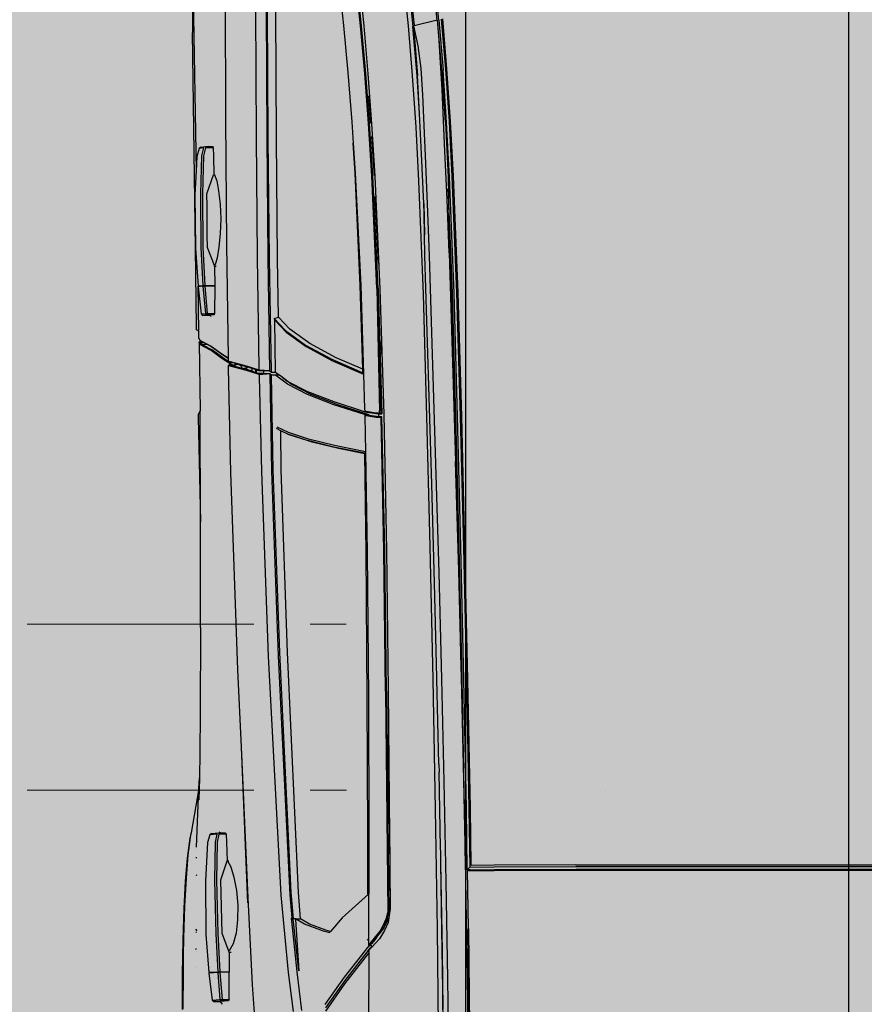
# Model space of a CAD drawing. Units: inches. Extents: x 1884 to 2398, y 474 to 1488.
# Tile 10 of 39: x 2186 to 2231, y 620 to 672. Entities that reach past the tile are written whole.
import ezdxf

# ---------------------------------------------------------------- set-up
doc = ezdxf.new("R2010")
doc.units = ezdxf.units.IN
doc.header["$MEASUREMENT"] = 0
doc.linetypes.add('ACAD_ISO02W100', pattern=[15, 12, -3])
doc.layers.get('0').update_dxf_attribs({"color": 250})
for name, color, linetype, lineweight in [('A-ANNO-DIMS', 2, 'Continuous', 18), ('A-FLOR-OVHD', 8, 'ACAD_ISO02W100', 18), ('C-VEHI', 8, 'Continuous', 18)]:
    doc.layers.add(name, color=color, linetype=linetype, lineweight=lineweight)
doc.layers.add('Edges', color=250, linetype='Continuous')
doc.layers.add('L-PVMT-PATT', color=9, linetype='Continuous', lineweight=13, true_color=0xc7c8ca)
doc.styles.get("Standard").update_dxf_attribs({"font": 'arial.ttf'})
doc.dimstyles.get("Standard").update_dxf_attribs({"dimtxt": 7, "dimasz": 0.18, "dimexe": 0.18, "dimexo": 0.0625, "dimgap": 0.09, "dimtad": 0, "dimtih": 1, "dimtoh": 1, "dimzin": 0, "dimdsep": 46, "dimlunit": 3, "dimtxsty": 'Standard', "dimcen": 0.09, "dimadec": 0, "dimazin": 0, "dimtfac": 1, "dimtofl": 0, "dimtmove": 0, "dimatfit": 3, "dimfxl": 1, "dimtolj": 1, "dimtzin": 0, "dimarcsym": 0})

# ---------------------------------------------------------------- blocks, each defined once
blk = doc.blocks.new('Nissan Qashqai pl')
at = {"layer": 'Edges'}
for p, q in [((10.4706, 11.5566), (10.4706, 12.2875)), ((10.4726, 11.5567), (10.4726, 12.2875)), ((10.4764, 11.5569), (10.4764, 12.2872)), ((10.4776, 11.5567), (10.4776, 12.2874)), ((10.4706, 11.5566), (10.4711, 11.4469)), ((10.4731, 11.4469), (10.4726, 11.5567)), ((10.4769, 11.4474), (10.4764, 11.5569)), ((10.4781, 11.4469), (10.4776, 11.5567)), ((10.4711, 11.4469), (10.4715, 11.416)), ((10.4735, 11.414), (10.4731, 11.4469)), ((10.4773, 11.4146), (10.4769, 11.4474)), ((10.4785, 11.4111), (10.4781, 11.4469)), ((10.4715, 11.416), (10.3947, 11.4148)), ((9.8673, 11.4031), (9.701, 11.3983)), ((10.0431, 11.4075), (9.8673, 11.4031)), ((9.8673, 11.4012), (10.043, 11.4055)), ((10.2215, 11.406), (10.0429, 11.4021)), ((10.2216, 11.4037), (10.0429, 11.3998)), ((10.043, 11.4055), (10.2218, 11.4094)), ((10.2218, 11.4114), (10.0431, 11.4075)), ((10.2043, 11.4025), (10.0747, 11.3991)), ((10.0998, 11.3999), (10.2043, 11.4025)), ((10.2175, 11.4028), (10.2043, 11.4025)), ((10.3564, 11.406), (10.2175, 11.4028)), ((10.3945, 11.4094), (10.2215, 11.406)), ((10.3947, 11.4071), (10.2216, 11.4037)), ((10.3947, 11.4148), (10.2218, 11.4114)), ((10.2218, 11.4094), (10.3947, 11.4128)), ((10.4416, 11.4077), (10.3564, 11.406)), ((10.4773, 11.4107), (10.3945, 11.4094)), ((10.3947, 11.4128), (10.4735, 11.414)), ((10.4416, 11.4078), (10.3947, 11.4071)), ((10.4519, 11.4079), (10.4416, 11.4077)), ((10.4519, 11.4079), (10.4416, 11.4078)), ((10.4416, 11.4077), (10.4416, 11.4078)), ((10.4524, 11.408), (10.4519, 11.4079)), ((10.4519, 11.4079), (10.4519, 11.4079)), ((10.4524, 11.4079), (10.4519, 11.4079)), ((10.4524, 11.4079), (10.4524, 11.408)), ((10.4533, 11.408), (10.4524, 11.408)), ((10.4533, 11.4079), (10.4524, 11.4079)), ((10.4638, 11.4081), (10.4533, 11.4079)), ((10.4638, 11.4081), (10.4533, 11.408)), ((10.4533, 11.4079), (10.4533, 11.408)), ((10.4914, 11.4087), (10.4638, 11.4081)), ((10.4773, 11.4107), (10.4735, 11.414)), ((10.4773, 11.4146), (10.4773, 11.4107)), ((10.4773, 11.4107), (10.5561, 11.4119)), ((10.4773, 11.4107), (10.4785, 11.4111)), ((10.5563, 11.4123), (10.4785, 11.4111)), ((10.6223, 11.4109), (10.4914, 11.4087)), ((10.6996, 11.4134), (10.5561, 11.4119)), ((10.5563, 11.4123), (10.6999, 11.4138)), ((10.7493, 11.4125), (10.6223, 11.4109)), ((9.5443, 11.3919), (9.4706, 11.388)), ((9.4709, 11.3861), (9.5446, 11.39)), ((9.701, 11.3983), (9.5443, 11.3919)), ((9.5446, 11.39), (9.7011, 11.3963)), ((9.7014, 11.3929), (9.5454, 11.3866)), ((9.7014, 11.3906), (9.5695, 11.3853)), ((9.6472, 11.3861), (9.9278, 11.3949)), ((9.6714, 11.3874), (9.8565, 11.3931)), ((9.7011, 11.3963), (9.8673, 11.4012)), ((9.8673, 11.3977), (9.7014, 11.3929)), ((9.8673, 11.3954), (9.7014, 11.3906)), ((9.8565, 11.3931), (9.9794, 11.3967)), ((10.0429, 11.4021), (9.8673, 11.3977)), ((10.0429, 11.3998), (9.8673, 11.3954)), ((10.0747, 11.3991), (9.9278, 11.3949)), ((9.9794, 11.3967), (10.0965, 11.3998)), ((10.0965, 11.3998), (10.0998, 11.3999)), ((9.4, 11.3832), (9.3326, 11.3776)), ((9.333, 11.3757), (9.4004, 11.3813)), ((9.4017, 11.3765), (9.3344, 11.3708)), ((9.3346, 11.3724), (9.4018, 11.378)), ((9.4276, 11.3767), (9.3918, 11.3747)), ((9.4706, 11.388), (9.4, 11.3832)), ((9.4004, 11.3813), (9.4709, 11.3861)), ((9.472, 11.3812), (9.4017, 11.3765)), ((9.472, 11.3828), (9.4018, 11.378)), ((9.4694, 11.3788), (9.4276, 11.3767)), ((9.5105, 11.3805), (9.4694, 11.3788)), ((9.5454, 11.3866), (9.472, 11.3828)), ((9.472, 11.3812), (9.5454, 11.3851)), ((9.5755, 11.3834), (9.5105, 11.3805)), ((9.5454, 11.3851), (9.5695, 11.3853)), ((9.5454, 11.3848), (9.5454, 11.3851)), ((9.5695, 11.3853), (9.5609, 11.3849)), ((9.5695, 11.3853), (9.5786, 11.3853)), ((9.6472, 11.3861), (9.5755, 11.3834)), ((9.5786, 11.3853), (9.6206, 11.3861)), ((9.6206, 11.3861), (9.6714, 11.3874)), ((10.0776, 11.3722), (10.2201, 11.3759)), ((10.2201, 11.3759), (10.3586, 11.3791)), ((10.3586, 11.3791), (10.4931, 11.3817)), ((10.5576, 11.3766), (10.4676, 11.3751)), ((10.5566, 11.3765), (10.4676, 11.3751)), ((10.5866, 11.3772), (10.4681, 11.3752)), ((10.4931, 11.3817), (10.6237, 11.3839)), ((10.5566, 11.3765), (10.7, 11.378)), ((10.6649, 11.3783), (10.5576, 11.3766)), ((10.6649, 11.3783), (10.5866, 11.3772)), ((10.6237, 11.3839), (10.7502, 11.3855)), ((9.3346, 11.3724), (9.2704, 11.3659)), ((9.3346, 11.37), (9.2724, 11.3637)), ((9.3611, 11.3727), (9.3344, 11.3708)), ((9.3344, 11.3708), (9.3346, 11.37)), ((9.3346, 11.37), (9.3418, 11.3391)), ((9.3918, 11.3747), (9.3611, 11.3727)), ((9.9583, 11.363), (9.651, 11.3536)), ((9.6514, 11.3592), (9.9312, 11.3681)), ((9.9312, 11.3681), (10.0776, 11.3722)), ((10.091, 11.3666), (9.9583, 11.363)), ((10.2211, 11.3646), (10.0423, 11.3607)), ((10.2191, 11.3699), (10.091, 11.3666)), ((10.2202, 11.3699), (10.2191, 11.3699)), ((10.2202, 11.3699), (10.2203, 11.3699)), ((10.3353, 11.3725), (10.2203, 11.3699)), ((10.3955, 11.368), (10.2211, 11.3646)), ((10.3353, 11.3725), (10.346, 11.3727)), ((10.4477, 11.3747), (10.346, 11.3727)), ((10.5572, 11.3704), (10.3955, 11.368)), ((10.4537, 11.3749), (10.4477, 11.3747)), ((10.4537, 11.3749), (10.4538, 11.3749)), ((10.4681, 11.3752), (10.4538, 11.3749)), ((10.4676, 11.3751), (10.4538, 11.3749)), ((10.4676, 11.3751), (10.4676, 11.3751)), ((10.7004, 11.372), (10.5572, 11.3704)), ((9.3992, 11.3482), (9.4347, 11.3502)), ((9.4347, 11.3502), (9.4761, 11.3522)), ((9.4761, 11.3522), (9.5168, 11.3539)), ((9.5811, 11.3522), (9.514, 11.3492)), ((9.5168, 11.3539), (9.5812, 11.3568)), ((9.7029, 11.3516), (9.5503, 11.3455)), ((9.5811, 11.3522), (9.6231, 11.3531)), ((9.594, 11.3527), (9.5811, 11.3522)), ((9.5812, 11.3568), (9.6514, 11.3592)), ((9.6231, 11.3531), (9.594, 11.3527)), ((9.651, 11.3536), (9.6231, 11.3531)), ((9.8673, 11.3563), (9.7029, 11.3516)), ((10.0423, 11.3607), (9.8673, 11.3563)), ((9.2789, 11.331), (9.3427, 11.3375)), ((9.2819, 11.333), (9.3418, 11.3391)), ((9.3418, 11.3391), (9.342, 11.3383)), ((9.342, 11.3383), (9.3687, 11.3441)), ((9.342, 11.3383), (9.4087, 11.3438)), ((9.4088, 11.3371), (9.3422, 11.3316)), ((9.4093, 11.3431), (9.3427, 11.3375)), ((9.3687, 11.3441), (9.3992, 11.3482)), ((9.4605, 11.3465), (9.4087, 11.3438)), ((9.4782, 11.3418), (9.4088, 11.3371)), ((9.4605, 11.3465), (9.4093, 11.3431)), ((9.514, 11.3492), (9.4605, 11.3465)), ((9.5503, 11.3455), (9.4782, 11.3418)), ((9.3422, 11.3316), (9.2783, 11.3251)), ((9.696, 11.2932), (9.8644, 11.2982)), ((9.8644, 11.2982), (10.0472, 11.3018)), ((10.0476, 11.2996), (9.8681, 11.2959)), ((10.0477, 11.2982), (9.869, 11.2946)), ((10.0472, 11.3018), (10.2357, 11.3043)), ((10.2367, 11.3022), (10.0476, 11.2996)), ((10.2369, 11.3008), (10.0477, 11.2982)), ((10.2357, 11.3043), (10.53, 11.3068)), ((10.2367, 11.3022), (10.5351, 11.305)), ((10.2369, 11.3008), (10.5348, 11.3036)), ((10.4153, 11.3058), (10.2954, 11.3046)), ((10.4153, 11.3058), (10.4174, 11.3058)), ((10.4174, 11.3058), (10.4181, 11.3058)), ((10.4181, 11.3058), (10.4182, 11.3058)), ((10.4182, 11.3058), (10.53, 11.3068)), ((10.53, 11.3068), (10.5301, 11.3068)), ((10.5301, 11.3068), (10.5323, 11.3065)), ((10.5323, 11.3065), (10.5419, 11.3051)), ((10.5422, 11.3021), (10.5348, 11.3036)), ((10.5424, 11.3035), (10.5351, 11.305)), ((10.5366, 11.3048), (10.536, 11.305)), ((10.5379, 11.3052), (10.5381, 11.305)), ((10.5419, 11.3051), (10.5463, 11.3031)), ((10.5419, 11.3051), (10.5479, 11.3042)), ((10.5522, 11.2977), (10.5422, 11.3021)), ((10.5472, 11.3014), (10.5424, 11.3035)), ((10.5463, 11.3031), (10.5551, 11.2984)), ((10.5546, 11.2982), (10.5472, 11.3014)), ((10.5479, 11.3042), (10.5589, 11.2991)), ((10.5598, 11.2935), (10.5522, 11.2977)), ((10.5583, 11.296), (10.5546, 11.2982)), ((10.5551, 11.2984), (10.5583, 11.296)), ((10.5589, 11.2991), (10.57, 11.2925)), ((9.5438, 11.2836), (9.4736, 11.2793)), ((9.4739, 11.282), (9.5443, 11.2863)), ((9.491, 11.2819), (9.5434, 11.2852)), ((9.6953, 11.2892), (9.5437, 11.2822)), ((9.6954, 11.2907), (9.5438, 11.2836)), ((9.5443, 11.2863), (9.696, 11.2932)), ((9.5717, 11.2865), (9.6618, 11.2907)), ((9.6953, 11.2892), (9.863, 11.2944)), ((9.6953, 11.2892), (9.8598, 11.2925)), ((9.6954, 11.2907), (9.8641, 11.2959)), ((9.7669, 11.2945), (9.7832, 11.2951)), ((9.8629, 11.2925), (9.8598, 11.2925)), ((9.8605, 11.2746), (9.8626, 11.2878)), ((9.8615, 11.2754), (9.8635, 11.2886)), ((9.8626, 11.2878), (9.8627, 11.2909)), ((9.8627, 11.2909), (9.8629, 11.2925)), ((9.8627, 11.2909), (9.8637, 11.291)), ((9.8629, 11.2925), (9.863, 11.2944)), ((9.8641, 11.2959), (9.863, 11.2944)), ((9.8635, 11.2886), (9.8637, 11.291)), ((9.8637, 11.291), (9.8638, 11.2934)), ((9.8637, 11.291), (9.8643, 11.291)), ((9.8638, 11.2934), (9.8641, 11.2959)), ((9.8643, 11.291), (9.8677, 11.291)), ((9.8675, 11.2887), (9.8655, 11.2754)), ((9.8686, 11.2879), (9.8665, 11.2747)), ((9.8677, 11.291), (9.8675, 11.2887)), ((9.8678, 11.2935), (9.8677, 11.291)), ((9.8681, 11.2959), (9.8678, 11.2935)), ((9.8681, 11.2959), (9.869, 11.2946)), ((9.8689, 11.2927), (9.8686, 11.2879)), ((9.869, 11.2946), (9.8689, 11.2927)), ((10.5612, 11.2944), (10.5583, 11.296)), ((10.5764, 11.28), (10.5598, 11.2935)), ((10.5683, 11.2885), (10.5612, 11.2944)), ((10.5683, 11.2885), (10.573, 11.285)), ((10.575, 11.2829), (10.5683, 11.2885)), ((10.57, 11.2925), (10.5811, 11.2822)), ((10.573, 11.285), (10.5769, 11.2818)), ((9.2801, 11.2648), (9.3418, 11.2713)), ((9.3418, 11.2713), (9.4064, 11.277)), ((9.4062, 11.2729), (9.3418, 11.2671)), ((9.4063, 11.2743), (9.3419, 11.2685)), ((9.4735, 11.2779), (9.4062, 11.2729)), ((9.4736, 11.2793), (9.4063, 11.2743)), ((9.4064, 11.277), (9.4739, 11.282)), ((9.4727, 11.2808), (9.4362, 11.278)), ((9.4727, 11.2808), (9.4732, 11.2808)), ((9.5437, 11.2822), (9.4735, 11.2779)), ((9.8039, 11.27), (9.6912, 11.2667)), ((9.6913, 11.2674), (9.8099, 11.2711)), ((9.8039, 11.27), (9.7884, 11.2343)), ((9.7905, 11.2283), (9.8087, 11.2702)), ((9.7925, 11.2294), (9.8107, 11.2711)), ((9.8087, 11.2702), (9.8039, 11.27)), ((9.8099, 11.2711), (9.8087, 11.2702)), ((9.8099, 11.2711), (9.8107, 11.2711)), ((9.8107, 11.2711), (9.8573, 11.2726)), ((9.8475, 11.2312), (9.8611, 11.2734)), ((9.8652, 11.2788), (9.8516, 11.2363)), ((9.8652, 11.2738), (9.8516, 11.2313)), ((9.8573, 11.2726), (9.8603, 11.2727)), ((9.8603, 11.2727), (9.8605, 11.2746)), ((9.8611, 11.2734), (9.8603, 11.2727)), ((9.8612, 11.2735), (9.8611, 11.2734)), ((9.8612, 11.2735), (9.8615, 11.2754)), ((9.8652, 11.2738), (9.8652, 11.2788)), ((9.8655, 11.2754), (9.8652, 11.2738)), ((9.8652, 11.2735), (9.8665, 11.2747)), ((9.8652, 11.2738), (9.8652, 11.2738)), ((9.8652, 11.2738), (9.8652, 11.2735)), ((9.8652, 11.2735), (9.8664, 11.2728)), ((9.8665, 11.2747), (9.8664, 11.2728)), ((9.8664, 11.2728), (9.9149, 11.2736)), ((9.9149, 11.2736), (9.9066, 11.2322)), ((9.9169, 11.2728), (9.9086, 11.2313)), ((9.9177, 11.2728), (9.9106, 11.2373)), ((9.9149, 11.2736), (10.0505, 11.276)), ((9.9177, 11.2728), (9.9169, 11.2728)), ((10.0501, 11.2747), (9.9177, 11.2728)), ((10.2453, 11.2762), (10.0501, 11.2747)), ((10.0505, 11.276), (10.2453, 11.2777)), ((10.2453, 11.2777), (10.4289, 11.2783)), ((10.4292, 11.2767), (10.2453, 11.2762)), ((10.4289, 11.2783), (10.5092, 11.2783)), ((10.5099, 11.2768), (10.4292, 11.2767)), ((10.5099, 11.2768), (10.5092, 11.2783)), ((10.5092, 11.2783), (10.5094, 11.2783)), ((10.5094, 11.2783), (10.51, 11.2776)), ((10.5783, 11.2783), (10.5094, 11.2783)), ((10.51, 11.2776), (10.5099, 11.2768)), ((10.51, 11.2776), (10.5419, 11.2423)), ((10.5705, 11.2771), (10.5709, 11.2767)), ((10.5709, 11.2767), (10.5719, 11.2759)), ((10.5776, 11.2808), (10.575, 11.2829)), ((10.5783, 11.2783), (10.5764, 11.28)), ((10.5796, 11.2787), (10.5776, 11.2808)), ((10.5776, 11.2808), (10.5783, 11.2783)), ((10.5796, 11.2787), (10.5783, 11.2783)), ((10.5796, 11.2824), (10.5796, 11.2787)), ((10.6215, 11.2456), (10.5796, 11.2787)), ((10.5811, 11.2822), (10.5821, 11.2808)), ((10.5811, 11.2822), (10.5834, 11.28)), ((10.5821, 11.2808), (10.5834, 11.2793)), ((10.5825, 11.2806), (10.5834, 11.2793)), ((10.5834, 11.28), (10.5851, 11.2783)), ((10.5834, 11.2793), (10.5835, 11.2793)), ((10.5835, 11.2793), (10.584, 11.2787)), ((10.584, 11.2789), (10.584, 11.2793)), ((10.584, 11.2787), (10.584, 11.2789)), ((10.584, 11.2787), (10.6261, 11.2458)), ((10.584, 11.2787), (10.5851, 11.2783)), ((10.5843, 11.2787), (10.584, 11.2787)), ((10.5847, 11.2787), (10.5843, 11.2787)), ((10.5851, 11.2783), (10.5892, 11.2783)), ((10.6306, 11.2459), (10.5892, 11.2783)), ((10.5892, 11.2783), (10.6988, 11.2779)), ((9.3418, 11.2671), (9.2803, 11.2606)), ((9.3419, 11.2685), (9.2804, 11.262)), ((9.471, 11.2554), (9.4997, 11.2573)), ((9.4997, 11.2573), (9.5403, 11.26)), ((9.5404, 11.2598), (9.4997, 11.2573)), ((9.5403, 11.26), (9.6913, 11.2674)), ((9.6912, 11.2667), (9.5404, 11.2598)), ((9.2814, 11.2377), (9.3416, 11.2442)), ((9.3416, 11.2442), (9.4048, 11.2501)), ((9.4048, 11.2501), (9.471, 11.2554)), ((10.6583, 11.2197), (10.6215, 11.2456)), ((10.6261, 11.2458), (10.6627, 11.22)), ((10.6671, 11.2203), (10.6306, 11.2459)), ((9.7884, 11.2343), (9.7692, 11.1989)), ((9.8338, 11.1956), (9.8475, 11.2312)), ((9.8516, 11.2363), (9.8378, 11.2007)), ((9.8516, 11.2313), (9.8378, 11.1957)), ((9.9066, 11.2322), (9.8978, 11.197)), ((9.9086, 11.2313), (9.8998, 11.196)), ((9.9106, 11.2373), (9.9018, 11.2021)), ((10.5419, 11.2423), (10.56, 11.2265)), ((9.7713, 11.1929), (9.7905, 11.2283)), ((9.7733, 11.194), (9.7925, 11.2294)), ((10.5584, 11.2206), (10.5502, 11.1986)), ((10.56, 11.2265), (10.5584, 11.2206)), ((10.5584, 11.2136), (10.5617, 11.2251)), ((10.56, 11.2265), (10.5617, 11.2251)), ((10.5584, 11.2136), (10.5502, 11.1916)), ((9.7692, 11.1989), (9.7499, 11.1721)), ((9.7519, 11.1661), (9.7713, 11.1929)), ((9.754, 11.1672), (9.7733, 11.194)), ((9.8201, 11.1685), (9.8338, 11.1956)), ((9.8378, 11.2007), (9.8241, 11.1736)), ((9.8378, 11.1957), (9.8241, 11.1686)), ((9.8978, 11.197), (9.8891, 11.1701)), ((9.8911, 11.1693), (9.8998, 11.196)), ((9.9018, 11.2021), (9.8931, 11.1752)), ((10.5502, 11.1986), (10.543, 11.1865)), ((10.5502, 11.1916), (10.543, 11.1795)), ((10.5079, 11.1835), (10.1849, 11.1687)), ((10.543, 11.1865), (10.5079, 11.1835)), ((10.543, 11.1795), (10.543, 11.1865)), ((10.5439, 11.1796), (10.543, 11.1795)), ((10.543, 11.1795), (10.543, 11.1771)), ((10.5439, 11.1796), (10.613, 11.1841)), ((10.5458, 11.1742), (10.6144, 11.1813)), ((10.613, 11.1841), (10.547, 11.1767)), ((10.6144, 11.1813), (10.6664, 11.1875)), ((9.7499, 11.1721), (9.7337, 11.1566)), ((9.7357, 11.1507), (9.7519, 11.1661)), ((9.7378, 11.1517), (9.754, 11.1672)), ((9.8241, 11.1686), (9.8119, 11.1529)), ((9.8241, 11.1736), (9.8147, 11.1616)), ((9.8147, 11.1616), (9.8201, 11.1685)), ((9.8891, 11.1701), (9.8818, 11.1551)), ((9.8911, 11.1691), (9.8867, 11.16)), ((9.8931, 11.1751), (9.8911, 11.1693)), ((9.8911, 11.1693), (9.8911, 11.1691)), ((9.8931, 11.1751), (9.8931, 11.1752)), ((10.1849, 11.1687), (9.9393, 11.1602)), ((10.5079, 11.1739), (10.1849, 11.1585)), ((10.1894, 11.1563), (10.5109, 11.1721)), ((10.543, 11.1771), (10.5079, 11.1739)), ((10.5109, 11.1721), (10.5417, 11.1748)), ((10.6152, 11.1702), (10.5113, 11.1603)), ((10.543, 11.1771), (10.5417, 11.1748)), ((10.5417, 11.1748), (10.5427, 11.1739)), ((10.5436, 11.1754), (10.5427, 11.1739)), ((10.5427, 11.1739), (10.5458, 11.1742)), ((10.544, 11.1763), (10.543, 11.1771)), ((10.544, 11.1763), (10.5436, 11.1754)), ((10.547, 11.1767), (10.544, 11.1763)), ((10.6678, 11.177), (10.6152, 11.1702)), ((9.4936, 11.1538), (9.3225, 11.1531)), ((9.6552, 11.1554), (9.4936, 11.1538)), ((9.7337, 11.1566), (9.6552, 11.1554)), ((9.7357, 11.1507), (9.7337, 11.1566)), ((9.7357, 11.1507), (9.7378, 11.1517)), ((9.8078, 11.1528), (9.7378, 11.1517)), ((9.8078, 11.1528), (9.8119, 11.1579)), ((9.8078, 11.1471), (9.8078, 11.1528)), ((9.8147, 11.1616), (9.8119, 11.1579)), ((9.8119, 11.1579), (9.8119, 11.1529)), ((9.8119, 11.1529), (9.8119, 11.1472)), ((9.8147, 11.1616), (9.8147, 11.1616)), ((9.8867, 11.16), (9.8838, 11.1541)), ((9.9393, 11.1602), (9.8867, 11.16)), ((10.1849, 11.1585), (9.9393, 11.1497)), ((9.9411, 11.1475), (10.1894, 11.1563)), ((10.5113, 11.1603), (10.19, 11.1433)), ((9.3198, 11.1403), (9.4922, 11.1409)), ((9.4936, 11.1428), (9.3225, 11.1421)), ((9.4922, 11.1409), (9.654, 11.1423)), ((9.6552, 11.1445), (9.4936, 11.1428)), ((9.654, 11.1423), (9.8061, 11.1447)), ((9.8078, 11.1471), (9.6552, 11.1445)), ((9.8061, 11.1447), (9.8051, 11.1309)), ((9.8058, 11.1369), (9.8061, 11.1447)), ((9.8061, 11.1447), (9.8078, 11.1471)), ((9.8101, 11.1449), (9.8098, 11.1369)), ((9.8101, 11.1449), (9.9411, 11.1475)), ((9.8119, 11.1472), (9.8101, 11.1449)), ((9.8101, 11.1449), (9.8112, 11.1311)), ((9.9393, 11.1497), (9.8119, 11.1472)), ((10.19, 11.1433), (9.9414, 11.1341)), ((9.4919, 11.1269), (9.3194, 11.1262)), ((9.6538, 11.1284), (9.4919, 11.1269)), ((9.802, 11.1309), (9.6538, 11.1284)), ((9.7992, 11.1133), (9.8044, 11.129)), ((9.8051, 11.1309), (9.802, 11.1309)), ((9.8026, 11.1212), (9.8041, 11.1256)), ((9.8041, 11.1256), (9.8045, 11.1268)), ((9.8041, 11.1256), (9.8081, 11.1256)), ((9.8044, 11.129), (9.8051, 11.1309)), ((9.8045, 11.1268), (9.8046, 11.1271)), ((9.8045, 11.1268), (9.8085, 11.1268)), ((9.8046, 11.1271), (9.8055, 11.1298)), ((9.8086, 11.1271), (9.8046, 11.1271)), ((9.8106, 11.1292), (9.8054, 11.1135)), ((9.8055, 11.1298), (9.8058, 11.1369)), ((9.8098, 11.1369), (9.8058, 11.1369)), ((9.8081, 11.1256), (9.8067, 11.1213)), ((9.8085, 11.1268), (9.8081, 11.1256)), ((9.8086, 11.1271), (9.8085, 11.1268)), ((9.8096, 11.13), (9.8086, 11.1271)), ((9.8098, 11.1369), (9.8096, 11.13)), ((9.8112, 11.1311), (9.8106, 11.1292)), ((9.8143, 11.1312), (9.8112, 11.1311)), ((9.9414, 11.1341), (9.8143, 11.1312)), ((10.6318, 11.1213), (10.6955, 11.1257)), ((9.7937, 11.0918), (9.7992, 11.1133)), ((9.7987, 11.108), (9.8002, 11.1141)), ((9.8054, 11.1135), (9.7999, 11.0919)), ((9.8002, 11.1141), (9.8008, 11.1157)), ((9.8008, 11.1157), (9.8014, 11.1176)), ((9.8014, 11.1139), (9.8008, 11.1157)), ((9.803, 11.1212), (9.8014, 11.1176)), ((9.8014, 11.1176), (9.8026, 11.1212)), ((9.8043, 11.1139), (9.8014, 11.1139)), ((9.8031, 11.1093), (9.8014, 11.1139)), ((9.803, 11.1212), (9.8026, 11.1212)), ((9.8067, 11.1213), (9.803, 11.1212)), ((9.8043, 11.1139), (9.8031, 11.1093)), ((9.8044, 11.1142), (9.8043, 11.1139)), ((9.8067, 11.1213), (9.8044, 11.1142)), ((10.312, 11.1064), (10.5147, 11.1156)), ((10.312, 11.1064), (10.5214, 11.1149)), ((10.5147, 11.1156), (10.6318, 11.1213)), ((9.7964, 11.0988), (9.7943, 11.0907)), ((9.7964, 11.0988), (9.7973, 11.1023)), ((9.7964, 11.0988), (9.7992, 11.0966)), ((9.7973, 11.1023), (9.7977, 11.1042)), ((9.7977, 11.1033), (9.7973, 11.1023)), ((9.7973, 11.1023), (9.7977, 11.1011)), ((9.7987, 11.1053), (9.7977, 11.1033)), ((9.7977, 11.1042), (9.7978, 11.1044)), ((9.7977, 11.1042), (9.7977, 11.1033)), ((9.7977, 11.1011), (9.7977, 11.0998)), ((9.7977, 11.1011), (9.7985, 11.099)), ((9.7977, 11.0998), (9.7985, 11.099)), ((9.7978, 11.1044), (9.7987, 11.108)), ((9.7987, 11.1053), (9.7978, 11.1044)), ((9.7985, 11.099), (9.7989, 11.098)), ((9.7992, 11.1065), (9.7987, 11.108)), ((9.7992, 11.1065), (9.7987, 11.1053)), ((9.7989, 11.098), (9.7998, 11.0976)), ((9.8027, 11.1078), (9.7992, 11.1065)), ((9.8002, 11.098), (9.7996, 11.0966)), ((9.8003, 11.0983), (9.7998, 11.0976)), ((9.8002, 11.098), (9.8001, 11.0974)), ((9.8003, 11.0983), (9.8002, 11.098)), ((9.8027, 11.1078), (9.8003, 11.0983)), ((9.8031, 11.1093), (9.8027, 11.1078)), ((9.9426, 11.0923), (10.2081, 11.1017)), ((10.2081, 11.1017), (10.312, 11.1064)), ((10.4871, 11.0967), (10.5048, 11.1002)), ((10.5048, 11.1002), (10.5246, 11.1019)), ((10.5246, 11.1019), (10.5445, 11.1017)), ((10.5445, 11.1017), (10.5625, 11.0996)), ((10.5625, 11.0996), (10.5769, 11.0957)), ((9.2886, 11.0848), (9.4673, 11.0852)), ((9.4673, 11.0852), (9.6358, 11.0866)), ((9.6358, 11.0866), (9.7887, 11.0889)), ((9.7832, 11.0805), (9.7887, 11.0889)), ((9.7842, 11.0814), (9.7891, 11.0889)), ((9.7933, 11.0892), (9.7883, 11.0815)), ((9.7887, 11.0889), (9.7891, 11.0889)), ((9.7891, 11.0889), (9.79, 11.0889)), ((9.7965, 11.0915), (9.7894, 11.0806)), ((9.79, 11.0889), (9.7931, 11.089)), ((9.7931, 11.089), (9.7934, 11.0906)), ((9.7931, 11.089), (9.7933, 11.0892)), ((9.7933, 11.0892), (9.7941, 11.0901)), ((9.7934, 11.0906), (9.7937, 11.0918)), ((9.7934, 11.0906), (9.7938, 11.0904)), ((9.7941, 11.0901), (9.7943, 11.0907)), ((9.7955, 11.0925), (9.7943, 11.0907)), ((9.7963, 11.0918), (9.7955, 11.0925)), ((9.7992, 11.0966), (9.7963, 11.0918)), ((9.7963, 11.0918), (9.7963, 11.0918)), ((9.7964, 11.0917), (9.7963, 11.0918)), ((9.7964, 11.0917), (9.7996, 11.0966)), ((9.7964, 11.0917), (9.7964, 11.0917)), ((9.7967, 11.0915), (9.7964, 11.0917)), ((9.7965, 11.0915), (9.7967, 11.0915)), ((9.7983, 11.0901), (9.7965, 11.0915)), ((9.7967, 11.0915), (9.7986, 11.0916)), ((9.7977, 11.0907), (9.7967, 11.0915)), ((9.7982, 11.0902), (9.7977, 11.0907)), ((9.7986, 11.0916), (9.7982, 11.0902)), ((9.7983, 11.0901), (9.7982, 11.0902)), ((9.7986, 11.0898), (9.7983, 11.0901)), ((9.7988, 11.0925), (9.7986, 11.0916)), ((9.7986, 11.0898), (9.7993, 11.0891)), ((9.7998, 11.0964), (9.7988, 11.0925)), ((9.7998, 11.0976), (9.7992, 11.0966)), ((9.7999, 11.0919), (9.7993, 11.0891)), ((9.7993, 11.0891), (9.8024, 11.0892)), ((9.8001, 11.0974), (9.7996, 11.0966)), ((9.7996, 11.0966), (9.7998, 11.0964)), ((9.8001, 11.0974), (9.7998, 11.0964)), ((9.8024, 11.0892), (9.9426, 11.0923)), ((10.4274, 11.0767), (10.4275, 11.0856)), ((10.4275, 11.0856), (10.4293, 11.0863)), ((10.4293, 11.0863), (10.4291, 11.0765)), ((10.4293, 11.0863), (10.4398, 11.0868)), ((10.4398, 11.0868), (10.4653, 11.0878)), ((10.4653, 11.0881), (10.4652, 11.0897)), ((10.4653, 11.0881), (10.4732, 11.0925)), ((10.4653, 11.0877), (10.4653, 11.0881)), ((10.4653, 11.0878), (10.4653, 11.0881)), ((10.4653, 11.0881), (10.4653, 11.0881)), ((10.4653, 11.0877), (10.4653, 11.0878)), ((10.4908, 11.0793), (10.4653, 11.0877)), ((10.4732, 11.0925), (10.4871, 11.0967)), ((10.5867, 11.0897), (10.563, 11.0809)), ((10.5769, 11.0957), (10.5863, 11.0904)), ((10.5863, 11.0904), (10.5867, 11.0897)), ((10.5885, 11.0904), (10.5867, 11.0897)), ((10.5885, 11.0931), (10.5885, 11.0904)), ((10.5885, 11.0904), (10.6141, 11.0905)), ((10.6141, 11.0905), (10.615, 11.0905)), ((10.6142, 11.0782), (10.6141, 11.0905)), ((10.6517, 11.0902), (10.615, 11.0905)), ((10.615, 11.0905), (10.6151, 11.0782)), ((10.6518, 11.0808), (10.6517, 11.0902)), ((10.6517, 11.0902), (10.6535, 11.0895)), ((10.6535, 11.0895), (10.6543, 11.0786)), ((10.6535, 11.0895), (10.6536, 11.0803)), ((9.5422, 11.0706), (9.5422, 11.0716)), ((9.5424, 11.0707), (9.5503, 11.0736)), ((9.5503, 11.0736), (9.5641, 11.076)), ((9.5641, 11.076), (9.5818, 11.0782)), ((9.5818, 11.0782), (9.6016, 11.0791)), ((9.6016, 11.0791), (9.6215, 11.0782)), ((9.6215, 11.0782), (9.6395, 11.0766)), ((9.6395, 11.0766), (9.654, 11.0744)), ((9.654, 11.0744), (9.6633, 11.0715)), ((9.6633, 11.0715), (9.6645, 11.0705)), ((9.6655, 11.0728), (9.6655, 11.0708)), ((9.7728, 11.066), (9.7832, 11.0805)), ((9.7738, 11.067), (9.7842, 11.0814)), ((9.7883, 11.0815), (9.7778, 11.0671)), ((9.7894, 11.0806), (9.7788, 11.0661)), ((10.4263, 11.0777), (10.4274, 11.0767)), ((10.4274, 11.0762), (10.4274, 11.0767)), ((10.4282, 11.0666), (10.4274, 11.0762)), ((10.4291, 11.0765), (10.4398, 11.0741)), ((10.4398, 11.0718), (10.4291, 11.0741)), ((10.4291, 11.0741), (10.4299, 11.0644)), ((10.4398, 11.0741), (10.4909, 11.0734)), ((10.4909, 11.0711), (10.4398, 11.0718)), ((10.563, 11.0809), (10.4908, 11.0793)), ((10.4909, 11.0734), (10.563, 11.075)), ((10.5631, 11.0727), (10.4909, 11.0711)), ((10.563, 11.075), (10.6142, 11.0779)), ((10.6142, 11.0756), (10.5631, 11.0727)), ((10.6142, 11.0779), (10.6142, 11.0782)), ((10.6142, 11.0765), (10.6142, 11.0779)), ((10.615, 11.0765), (10.6142, 11.0765)), ((10.6142, 11.0756), (10.6142, 11.0765)), ((10.615, 11.0639), (10.6142, 11.0756)), ((10.6151, 11.0765), (10.615, 11.0765)), ((10.615, 11.0765), (10.6151, 11.0639)), ((10.6151, 11.078), (10.6518, 11.0808)), ((10.6518, 11.0784), (10.6151, 11.0756)), ((10.6151, 11.0782), (10.6151, 11.078)), ((10.6151, 11.078), (10.6151, 11.0765)), ((10.6151, 11.0765), (10.6151, 11.0756)), ((10.6151, 11.0756), (10.616, 11.0629)), ((10.6518, 11.0784), (10.6518, 11.0808)), ((10.6518, 11.0808), (10.6536, 11.0803)), ((10.6536, 11.0803), (10.6518, 11.0784)), ((10.6526, 11.0674), (10.6518, 11.0784)), ((10.6536, 11.0803), (10.6537, 11.0783)), ((10.6543, 11.0786), (10.6537, 11.0783)), ((10.6537, 11.0783), (10.6543, 11.0693)), ((10.6578, 11.0814), (10.6543, 11.0786)), ((10.6543, 11.0693), (10.6543, 11.0786)), ((9.5037, 11.0635), (9.5045, 11.0628)), ((9.5044, 11.0586), (9.5045, 11.0628)), ((9.5052, 11.0524), (9.5044, 11.0586)), ((9.5045, 11.0683), (9.5063, 11.0687)), ((9.5045, 11.0628), (9.5045, 11.0683)), ((9.5063, 11.0687), (9.5061, 11.0586)), ((9.5061, 11.0586), (9.5167, 11.0559)), ((9.5063, 11.0687), (9.5168, 11.0691)), ((9.5168, 11.0691), (9.5423, 11.0696)), ((9.5422, 11.0706), (9.5424, 11.0707)), ((9.5423, 11.0696), (9.5422, 11.0706)), ((9.5426, 11.0695), (9.5423, 11.0696)), ((9.5426, 11.0695), (9.5424, 11.0707)), ((9.5667, 11.0609), (9.5426, 11.0695)), ((9.5678, 11.0604), (9.5667, 11.0609)), ((9.5846, 11.0606), (9.5678, 11.0604)), ((9.6236, 11.0609), (9.5846, 11.0606)), ((9.64, 11.0611), (9.6236, 11.0609)), ((9.6413, 11.0616), (9.64, 11.0611)), ((9.6645, 11.0705), (9.6413, 11.0616)), ((9.6655, 11.0708), (9.6645, 11.0705)), ((9.6655, 11.0708), (9.6911, 11.0709)), ((9.6911, 11.0709), (9.692, 11.0709)), ((9.6911, 11.0645), (9.6911, 11.0709)), ((9.6912, 11.0631), (9.6911, 11.0645)), ((9.692, 11.0631), (9.6912, 11.0631)), ((9.6912, 11.0577), (9.6912, 11.0631)), ((9.692, 11.0709), (9.692, 11.0645)), ((9.692, 11.0709), (9.7287, 11.0708)), ((9.692, 11.0645), (9.692, 11.0631)), ((9.692, 11.0631), (9.6921, 11.0578)), ((9.6921, 11.0578), (9.7288, 11.0609)), ((9.7288, 11.0588), (9.6922, 11.0556)), ((9.7287, 11.0708), (9.7305, 11.0704)), ((9.7288, 11.0609), (9.7287, 11.0708)), ((9.7288, 11.0588), (9.7288, 11.0609)), ((9.7288, 11.0609), (9.7306, 11.0607)), ((9.7306, 11.0607), (9.7288, 11.0588)), ((9.7296, 11.0527), (9.7288, 11.0588)), ((9.7305, 11.0704), (9.7313, 11.0644)), ((9.7305, 11.0704), (9.7306, 11.0607)), ((9.7306, 11.0607), (9.7314, 11.0547)), ((9.733, 11.066), (9.7313, 11.0644)), ((9.7314, 11.0547), (9.7313, 11.0644)), ((9.7674, 11.0557), (9.7728, 11.066)), ((9.7684, 11.0567), (9.7717, 11.0631)), ((9.7717, 11.0631), (9.7707, 11.0593)), ((9.7707, 11.0593), (9.7709, 11.0549)), ((9.7717, 11.0631), (9.7738, 11.067)), ((9.7778, 11.0671), (9.7724, 11.0568)), ((9.7788, 11.0661), (9.7734, 11.0558)), ((10.4282, 11.0666), (10.4299, 11.0644)), ((10.4299, 11.0644), (10.4406, 11.0612)), ((10.4406, 11.0612), (10.4919, 11.0584)), ((10.4919, 11.0584), (10.564, 11.0591)), ((10.564, 11.0591), (10.6151, 11.0628)), ((10.6151, 11.0639), (10.615, 11.0639)), ((10.6151, 11.0628), (10.615, 11.0639)), ((10.6151, 11.0639), (10.6151, 11.0628)), ((10.616, 11.0629), (10.6526, 11.0674)), ((10.6526, 11.0674), (10.6543, 11.0693)), ((9.2517, 11.0411), (9.5372, 11.0459)), ((9.641, 11.045), (9.351, 11.0411)), ((9.5052, 11.0524), (9.5069, 11.0501)), ((9.5168, 11.0537), (9.5061, 11.0564)), ((9.5061, 11.0564), (9.5069, 11.0501)), ((9.5069, 11.0501), (9.5176, 11.0469)), ((9.5167, 11.0559), (9.5679, 11.0543)), ((9.5679, 11.0521), (9.5168, 11.0537)), ((9.5176, 11.0469), (9.5372, 11.0459)), ((9.5372, 11.0459), (9.5689, 11.0442)), ((9.5679, 11.0543), (9.64, 11.0549)), ((9.6401, 11.0528), (9.5679, 11.0521)), ((9.5689, 11.0442), (9.641, 11.045)), ((9.64, 11.0549), (9.6912, 11.0577)), ((9.6913, 11.0556), (9.6401, 11.0528)), ((9.641, 11.045), (9.6921, 11.0485)), ((9.7466, 11.0464), (9.641, 11.045)), ((9.6913, 11.0556), (9.6912, 11.0577)), ((9.692, 11.0499), (9.6913, 11.0556)), ((9.6922, 11.0499), (9.692, 11.0499)), ((9.6921, 11.0485), (9.692, 11.0499)), ((9.6922, 11.0556), (9.6921, 11.0578)), ((9.6922, 11.0499), (9.6921, 11.0485)), ((9.7526, 11.0495), (9.6921, 11.0485)), ((9.6922, 11.0556), (9.693, 11.0486)), ((9.6922, 11.0556), (9.6922, 11.0499)), ((9.693, 11.0486), (9.7296, 11.0527)), ((9.7296, 11.0527), (9.7314, 11.0547)), ((9.7511, 11.0463), (9.7466, 11.0464)), ((9.7526, 11.0495), (9.7511, 11.0463)), ((9.7623, 11.0497), (9.7526, 11.0495)), ((9.7623, 11.0497), (9.7643, 11.0504)), ((9.7643, 11.0504), (9.7652, 11.0514)), ((9.7643, 11.0504), (9.7648, 11.0513)), ((9.7648, 11.0513), (9.7664, 11.054)), ((9.7648, 11.0513), (9.7648, 11.0513)), ((9.7652, 11.0514), (9.7665, 11.0535)), ((9.7664, 11.054), (9.7674, 11.0557)), ((9.7665, 11.0537), (9.7664, 11.054)), ((9.7665, 11.0535), (9.7676, 11.0553)), ((9.7667, 11.0508), (9.7665, 11.0535)), ((9.7676, 11.0511), (9.7667, 11.0508)), ((9.7677, 11.0498), (9.7667, 11.0508)), ((9.7673, 11.0545), (9.7676, 11.0553)), ((9.7673, 11.0543), (9.7673, 11.0545)), ((9.7676, 11.0511), (9.7673, 11.0543)), ((9.7676, 11.0553), (9.7684, 11.0567)), ((9.7676, 11.0555), (9.7678, 11.056)), ((9.769, 11.0516), (9.7676, 11.0511)), ((9.7677, 11.0498), (9.8598, 11.0514)), ((9.77, 11.0506), (9.7677, 11.0498)), ((9.7677, 11.0498), (9.7677, 11.0498)), ((9.7712, 11.055), (9.769, 11.0516)), ((9.7734, 11.0558), (9.77, 11.0506)), ((9.7709, 11.0549), (9.7712, 11.055)), ((9.7724, 11.0568), (9.7712, 11.055)), ((9.8598, 11.0514), (9.8614, 11.0504)), ((9.8643, 11.0514), (9.8598, 11.0514)), ((9.8614, 11.0504), (9.8647, 11.0485)), ((10.0085, 11.0519), (9.8643, 11.0514)), ((9.8647, 11.0485), (9.869, 11.0488)), ((9.869, 11.0488), (10.0085, 11.0519)), ((10.0124, 11.0519), (10.0085, 11.0519)), ((10.1513, 11.0517), (10.0124, 11.0519)), ((10.1513, 11.0517), (10.2677, 11.0512)), ((10.2677, 11.0512), (10.3189, 11.0511)), ((10.3189, 11.0511), (10.3537, 11.0503)), ((10.3537, 11.0503), (10.3832, 11.0496)), ((10.3679, 11.0497), (10.3537, 11.0503)), ((10.3679, 11.0497), (10.4275, 11.0391)), ((10.4468, 11.0466), (10.3679, 11.0497)), ((10.4502, 11.0466), (10.4503, 11.0465)), ((10.4613, 11.0464), (10.4603, 11.0465)), ((10.4838, 11.0465), (10.4852, 11.046)), ((10.5565, 11.0456), (10.5591, 11.0464)), ((10.5615, 11.0464), (10.5617, 11.0457)), ((10.583, 11.0457), (10.5835, 11.0461)), ((10.5836, 11.0461), (10.5832, 11.0457)), ((10.5847, 11.0461), (10.5841, 11.0457)), ((10.5873, 11.0461), (10.5873, 11.0461)), ((10.6087, 11.0458), (10.6087, 11.0458)), ((9.2517, 11.0411), (9.351, 11.0411)), ((10.4275, 11.0391), (10.4304, 11.0385)), ((10.4304, 11.0385), (10.4339, 11.0381)), ((10.4345, 11.0379), (10.4339, 11.0381)), ((10.4339, 11.0381), (10.4573, 11.0349)), ((10.4613, 11.0343), (10.4345, 11.0379)), ((10.4573, 11.0349), (10.4889, 11.0323)), ((10.4926, 11.0317), (10.4613, 11.0343)), ((10.4889, 11.0323), (10.526, 11.0304)), ((10.5294, 11.0298), (10.4926, 11.0317)), ((10.526, 11.0304), (10.569, 11.0291)), ((10.5719, 11.0285), (10.5294, 11.0298)), ((10.569, 11.0291), (10.5919, 11.0287)), ((10.6176, 11.0277), (10.5719, 11.0285)), ((10.5919, 11.0287), (10.5936, 11.0286)), ((10.5936, 11.0286), (10.6151, 11.0283)), ((10.6151, 11.0283), (10.6644, 11.028)), ((10.6651, 11.0274), (10.6176, 11.0277))]:
    blk.add_line(p, q, dxfattribs=at)
blk = doc.blocks.new('car')
blk.add_blockref('Nissan Qashqai pl', (-9.7433, -11.9151))
blk = doc.blocks.new('carr')
blk.add_blockref('car', (0.5124, -0.007))
blk = doc.blocks.new('*D44')
at = {"layer": 'A-ANNO-DIMS', "color": 0, "lineweight": -2, "transparency": 16777216}
for p, q in [((2209.755, 1247.822), (2209.755, 484.005)), ((2230.029, 1247.822), (2230.029, 484.005)), ((2209.935, 484.185), (2229.849, 484.185)), ((2230.029, 484.185), (2230.209, 484.185))]:
    blk.add_line(p, q, dxfattribs=at)
at = {"layer": 'A-ANNO-DIMS', "color": 0, "lineweight": 100, "transparency": 16777216}
for points in [[(2209.935, 484.215), (2209.935, 484.155), (2209.755, 484.185)], [(2229.849, 484.215), (2229.849, 484.155), (2230.029, 484.185)]]:
    blk.add_solid(points, dxfattribs=at)
at = {"layer": 'Defpoints', "color": 0, "lineweight": 100, "transparency": 16777216}
for p in [(2209.755, 1247.885), (2230.029, 1247.885), (2230.029, 484.185)]:
    blk.add_point(p, dxfattribs=at)
at = {"layer": 'A-ANNO-DIMS', "color": 0, "transparency": 16777216, "insert": (2247.429, 484.185), "char_height": 7, "attachment_point": 5}
blk.add_mtext('\\A1;1\'-8 1/2"', dxfattribs=at)

msp = doc.modelspace()

# ---------------------------------------------------------------- hatches: boundary and pattern name
at = {"layer": 'L-PVMT-PATT'}
h = msp.add_hatch(color=256, dxfattribs=at)
h.dxf.hatch_style = 1
h.paths.add_polyline_path([(2387.529, 769.966), (2351.529, 769.966), (2238.447, 769.966), (2238.447, 762.15), (2238.447, 754.445), (2126.529, 754.445), (2126.529, 676.183), (2134.868, 676.183), (2142.673, 676.183), (2142.673, 646.578), (2134.868, 646.578), (2126.529, 646.578), (2126.529, 640.17), (2387.529, 640.17)])
h.paths.add_polyline_path([(2387.529, 631.385), (2303.086, 631.385), (2303.086, 615.671), (2387.529, 615.671)])
h.paths.add_polyline_path([(2387.529, 640.17), (2126.529, 640.17), (2126.529, 631.385), (2387.529, 631.385)])
h.paths.add_polyline_path([(2393.529, 604.13), (2387.529, 604.13), (2387.529, 615.671), (2303.086, 615.671), (2303.086, 607.943), (2249.649, 607.943), (2126.529, 607.943), (2126.529, 533.885), (2393.529, 533.885)])
h.paths.add_polyline_path([(2257.825, 611.008), (2257.83, 611.337), (2257.915, 616.493), (2258.021, 621.805), (2258.146, 627.274), (2258.252, 631.385), (2126.529, 631.385), (2126.529, 611.008)])
h.paths.add_polyline_path([(2258.892, 611.285), (2258.888, 611.008), (2300.247, 611.008), (2300.247, 631.385), (2259.314, 631.385), (2259.206, 627.173), (2259.081, 621.72), (2258.976, 616.424)])

# ---------------------------------------------------------------- linework, layer by layer
at = {"layer": 'A-FLOR-OVHD'}
for p, q in [((2126.529, 640.17), (2203.428, 640.17)), ((2126.529, 631.385), (2203.439, 631.385)), ((2217.153, 631.385), (2217.158, 631.385))]:
    msp.add_line(p, q, dxfattribs=at)

# ---------------------------------------------------------------- block references
at = {"layer": 'C-VEHI', "xscale": 39.37007874015748, "yscale": 39.37007874015748, "zscale": 39.37007874015748, "rotation": 270}
msp.add_blockref('carr', (2229.977, 676.232), dxfattribs=at)

# ---------------------------------------------------------------- dimensions: what is measured, and where the dimension line sits
at = {"layer": 'A-ANNO-DIMS'}
dim = msp.add_linear_dim(base=(2230.029, 484.185), p1=(2209.755, 1247.885), p2=(2230.029, 1247.885), dimstyle='Standard', override={"dimdec": 1, "dimlfac": 1, "dimrnd": 0, "dimzin": 1, "dimdsep": 46, "dimlunit": 4, "dimfrac": 2}, dxfattribs=at)
dim.commit()
dim.dimension.update_dxf_attribs({"geometry": '*D44', "text_midpoint": (2247.429, 484.185)})

doc.saveas('drawing.dxf')
